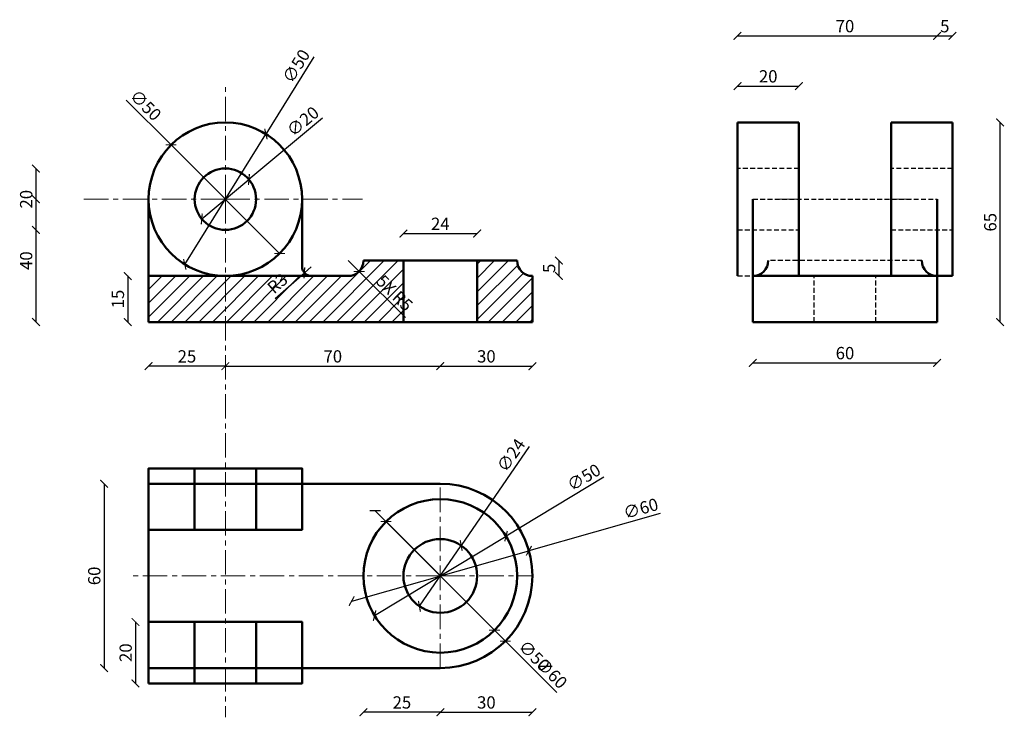
# Model space of a CAD drawing. Units: millimetres. Extents: x 2989 to 6790, y 1383 to 3069.
# Tile 1 of 1: x 2989.2 to 3309.8, y 1383.2 to 1610.3. Entities that reach past the tile are written whole.
import ezdxf

# ---------------------------------------------------------------- set-up
doc = ezdxf.new("R2010")
doc.units = ezdxf.units.MM
doc.header["$LTSCALE"] = 0.25
doc.linetypes.add('CENTER', pattern=[50.8, 31.75, -6.35, 6.35, -6.35])
doc.linetypes.add('HIDDEN', pattern=[9.525, 6.35, -3.175])
for name, color, linetype, lineweight in [('M-CNTR', 1, 'CENTER', 18), ('M-DIMS', 2, 'Continuous', 25), ('M-HATC', 8, 'Continuous', 18), ('M-HIDN', 6, 'HIDDEN', 25), ('M-OUTL', 7, 'Continuous', 50)]:
    doc.layers.add(name, color=color, linetype=linetype, lineweight=lineweight)
doc.styles.get("Standard").update_dxf_attribs({"font": 'arial.ttf'})
doc.dimstyles.new('ISO-25', dxfattribs={"dimtxt": 4, "dimasz": 2.5, "dimexe": 1.25, "dimexo": 0.625, "dimtad": 1, "dimdec": 0, "dimtxsty": 'Standard', "dimblk": 'ARCHTICK', "dimcen": 2.5, "dimse1": 1, "dimse2": 1, "dimadec": 0, "dimazin": 0, "dimtfac": 1, "dimtdec": 0, "dimtmove": 0, "dimatfit": 3, "dimfxl": 1, "dimarcsym": 0})

# ---------------------------------------------------------------- blocks, each defined once
blk = doc.blocks.new('_ArchTick')
at = {"color": 0, "linetype": 'ByBlock', "const_width": 0.15}
blk.add_lwpolyline([(-0.5, -0.5), (0.5, 0.5)], dxfattribs=at)
blk = doc.blocks.new('*D1')
at = {"layer": 'Defpoints', "color": 0, "transparency": 16777216}
for p in [(3126.13, 1429.2), (3156.13, 1429.2), (3156.13, 1384.81)]:
    blk.add_point(p, dxfattribs=at)
at = {"layer": 'M-DIMS', "color": 0, "lineweight": -2, "transparency": 16777216}
blk.add_line((3126.13, 1384.81), (3156.13, 1384.81), dxfattribs=at)
at = {"layer": 'M-DIMS', "color": 0, "lineweight": -2, "transparency": 16777216, "xscale": 2.5, "yscale": 2.5, "zscale": 2.5, "rotation": 180}
blk.add_blockref('_ArchTick', (3126.13, 1384.81), dxfattribs=at)
at = {"layer": 'M-DIMS', "color": 0, "lineweight": -2, "transparency": 16777216, "xscale": 2.5, "yscale": 2.5, "zscale": 2.5}
blk.add_blockref('_ArchTick', (3156.13, 1384.81), dxfattribs=at)
at = {"layer": 'M-DIMS', "color": 0, "transparency": 16777216, "insert": (3141.13, 1387.48), "char_height": 4, "attachment_point": 5}
blk.add_mtext('30', dxfattribs=at)
blk = doc.blocks.new('*D2')
at = {"layer": 'Defpoints', "color": 0, "transparency": 16777216}
for p in [(3126.13, 1511.85), (3156.13, 1511.85), (3156.13, 1497.49)]:
    blk.add_point(p, dxfattribs=at)
at = {"layer": 'M-DIMS', "color": 0, "lineweight": -2, "transparency": 16777216}
blk.add_line((3126.13, 1497.49), (3156.13, 1497.49), dxfattribs=at)
at = {"layer": 'M-DIMS', "color": 0, "lineweight": -2, "transparency": 16777216, "xscale": 2.5, "yscale": 2.5, "zscale": 2.5, "rotation": 180}
blk.add_blockref('_ArchTick', (3126.13, 1497.49), dxfattribs=at)
at = {"layer": 'M-DIMS', "color": 0, "lineweight": -2, "transparency": 16777216, "xscale": 2.5, "yscale": 2.5, "zscale": 2.5}
blk.add_blockref('_ArchTick', (3156.13, 1497.49), dxfattribs=at)
at = {"layer": 'M-DIMS', "color": 0, "transparency": 16777216, "insert": (3141.13, 1500.16), "char_height": 4, "attachment_point": 5}
blk.add_mtext('30', dxfattribs=at)
blk = doc.blocks.new('*D3')
at = {"layer": 'Defpoints', "color": 0, "transparency": 16777216}
for p in [(3031.13, 1511.85), (3056.13, 1511.85), (3031.13, 1497.49)]:
    blk.add_point(p, dxfattribs=at)
at = {"layer": 'M-DIMS', "color": 0, "lineweight": -2, "transparency": 16777216}
blk.add_line((3056.13, 1497.49), (3031.13, 1497.49), dxfattribs=at)
at = {"layer": 'M-DIMS', "color": 0, "lineweight": -2, "transparency": 16777216, "xscale": 2.5, "yscale": 2.5, "zscale": 2.5, "rotation": 180}
blk.add_blockref('_ArchTick', (3031.13, 1497.49), dxfattribs=at)
at = {"layer": 'M-DIMS', "color": 0, "lineweight": -2, "transparency": 16777216, "xscale": 2.5, "yscale": 2.5, "zscale": 2.5}
blk.add_blockref('_ArchTick', (3056.13, 1497.49), dxfattribs=at)
at = {"layer": 'M-DIMS', "color": 0, "transparency": 16777216, "insert": (3043.63, 1500.16), "char_height": 4, "attachment_point": 5}
blk.add_mtext('25', dxfattribs=at)
blk = doc.blocks.new('*D4')
at = {"layer": 'Defpoints', "color": 0, "transparency": 16777216}
for p in [(3056.13, 1511.85), (3126.13, 1511.85), (3126.13, 1497.49)]:
    blk.add_point(p, dxfattribs=at)
at = {"layer": 'M-DIMS', "color": 0, "lineweight": -2, "transparency": 16777216}
blk.add_line((3056.13, 1497.49), (3126.13, 1497.49), dxfattribs=at)
at = {"layer": 'M-DIMS', "color": 0, "lineweight": -2, "transparency": 16777216, "xscale": 2.5, "yscale": 2.5, "zscale": 2.5, "rotation": 180}
blk.add_blockref('_ArchTick', (3056.13, 1497.49), dxfattribs=at)
at = {"layer": 'M-DIMS', "color": 0, "lineweight": -2, "transparency": 16777216, "xscale": 2.5, "yscale": 2.5, "zscale": 2.5}
blk.add_blockref('_ArchTick', (3126.13, 1497.49), dxfattribs=at)
at = {"layer": 'M-DIMS', "color": 0, "transparency": 16777216, "insert": (3091.13, 1500.16), "char_height": 4, "attachment_point": 5}
blk.add_mtext('70', dxfattribs=at)
blk = doc.blocks.new('*D6')
at = {"layer": 'Defpoints', "color": 0, "transparency": 16777216}
for p in [(3101.13, 1429.2), (3126.13, 1429.2), (3101.13, 1384.81)]:
    blk.add_point(p, dxfattribs=at)
at = {"layer": 'M-DIMS', "color": 0, "lineweight": -2, "transparency": 16777216}
blk.add_line((3126.13, 1384.81), (3101.13, 1384.81), dxfattribs=at)
at = {"layer": 'M-DIMS', "color": 0, "lineweight": -2, "transparency": 16777216, "xscale": 2.5, "yscale": 2.5, "zscale": 2.5, "rotation": 180}
blk.add_blockref('_ArchTick', (3101.13, 1384.81), dxfattribs=at)
at = {"layer": 'M-DIMS', "color": 0, "lineweight": -2, "transparency": 16777216, "xscale": 2.5, "yscale": 2.5, "zscale": 2.5}
blk.add_blockref('_ArchTick', (3126.13, 1384.81), dxfattribs=at)
at = {"layer": 'M-DIMS', "color": 0, "transparency": 16777216, "insert": (3113.63, 1387.48), "char_height": 4, "attachment_point": 5}
blk.add_mtext('25', dxfattribs=at)
blk = doc.blocks.new('*D7')
at = {"layer": 'Defpoints', "color": 0, "transparency": 16777216}
for p in [(3138.13, 1540.69), (3114.13, 1531.85), (3138.13, 1531.85)]:
    blk.add_point(p, dxfattribs=at)
at = {"layer": 'M-DIMS', "color": 0, "lineweight": -2, "transparency": 16777216}
blk.add_line((3114.13, 1540.69), (3138.13, 1540.69), dxfattribs=at)
at = {"layer": 'M-DIMS', "color": 0, "lineweight": -2, "transparency": 16777216, "xscale": 2.5, "yscale": 2.5, "zscale": 2.5, "rotation": 180}
blk.add_blockref('_ArchTick', (3114.13, 1540.69), dxfattribs=at)
at = {"layer": 'M-DIMS', "color": 0, "lineweight": -2, "transparency": 16777216, "xscale": 2.5, "yscale": 2.5, "zscale": 2.5}
blk.add_blockref('_ArchTick', (3138.13, 1540.69), dxfattribs=at)
at = {"layer": 'M-DIMS', "color": 0, "transparency": 16777216, "insert": (3126.13, 1543.32), "char_height": 4, "attachment_point": 5}
blk.add_mtext('24', dxfattribs=at)
blk = doc.blocks.new('*D8')
at = {"layer": 'Defpoints', "color": 0, "transparency": 16777216}
for p in [(3063.81, 1558.26), (3048.45, 1545.44)]:
    blk.add_point(p, dxfattribs=at)
at = {"layer": 'M-DIMS', "color": 0, "lineweight": -2, "transparency": 16777216}
for p in [(3087.82, 1578.29), (3048.45, 1545.44)]:
    blk.add_line(p, (3063.81, 1558.26), dxfattribs=at)
at = {"layer": 'M-DIMS', "color": 0, "lineweight": -2, "transparency": 16777216, "xscale": 2.5, "yscale": 2.5, "zscale": 2.5}
for p, rotation in [((3063.81, 1558.26), 219.8399543782543), ((3048.45, 1545.44), 39.83995437825426)]:
    blk.add_blockref('_ArchTick', p, dxfattribs=dict(at, rotation=rotation))
at = {"layer": 'M-DIMS', "color": 0, "transparency": 16777216, "insert": (3081.69, 1576.8), "char_height": 4, "attachment_point": 5, "rotation": 39.84}
blk.add_mtext('∅20', dxfattribs=at)
blk = doc.blocks.new('*D9')
at = {"layer": 'Defpoints', "color": 0, "transparency": 16777216}
for p in [(3069.34, 1573.08), (3042.92, 1530.62)]:
    blk.add_point(p, dxfattribs=at)
at = {"layer": 'M-DIMS', "color": 0, "lineweight": -2, "transparency": 16777216}
for p in [(3084.99, 1598.24), (3042.92, 1530.62)]:
    blk.add_line(p, (3069.34, 1573.08), dxfattribs=at)
at = {"layer": 'M-DIMS', "color": 0, "lineweight": -2, "transparency": 16777216, "xscale": 2.5, "yscale": 2.5, "zscale": 2.5}
for p, rotation in [((3069.34, 1573.08), 238.1130736025114), ((3042.92, 1530.62), 58.11307360251142)]:
    blk.add_blockref('_ArchTick', p, dxfattribs=dict(at, rotation=rotation))
at = {"layer": 'M-DIMS', "color": 0, "transparency": 16777216, "insert": (3079.64, 1594.91), "char_height": 4, "attachment_point": 5, "rotation": 58.1131}
blk.add_mtext('∅50', dxfattribs=at)
blk = doc.blocks.new('*D10')
at = {"layer": 'Defpoints', "color": 0, "transparency": 16777216}
for p in [(3132.93, 1439.09), (3119.33, 1419.32)]:
    blk.add_point(p, dxfattribs=at)
at = {"layer": 'M-DIMS', "color": 0, "lineweight": -2, "transparency": 16777216}
for p in [(3155.09, 1471.29), (3119.33, 1419.32)]:
    blk.add_line(p, (3132.93, 1439.09), dxfattribs=at)
at = {"layer": 'M-DIMS', "color": 0, "lineweight": -2, "transparency": 16777216, "xscale": 2.5, "yscale": 2.5, "zscale": 2.5}
for p, rotation in [((3132.93, 1439.09), 235.4688788951653), ((3119.33, 1419.32), 55.46887889516527)]:
    blk.add_blockref('_ArchTick', p, dxfattribs=dict(at, rotation=rotation))
at = {"layer": 'M-DIMS', "color": 0, "transparency": 16777216, "insert": (3149.59, 1468.2), "char_height": 4, "attachment_point": 5, "rotation": 55.4689}
blk.add_mtext('∅24', dxfattribs=at)
blk = doc.blocks.new('*D11')
at = {"layer": 'Defpoints', "color": 0, "transparency": 16777216}
for p in [(3147.53, 1442.13), (3104.73, 1416.28)]:
    blk.add_point(p, dxfattribs=at)
at = {"layer": 'M-DIMS', "color": 0, "lineweight": -2, "transparency": 16777216}
for p in [(3179.41, 1461.38), (3104.73, 1416.28)]:
    blk.add_line(p, (3147.53, 1442.13), dxfattribs=at)
at = {"layer": 'M-DIMS', "color": 0, "lineweight": -2, "transparency": 16777216, "xscale": 2.5, "yscale": 2.5, "zscale": 2.5}
for p, rotation in [((3147.53, 1442.13), 211.1310054605087), ((3104.73, 1416.28), 31.13100546050863)]:
    blk.add_blockref('_ArchTick', p, dxfattribs=dict(at, rotation=rotation))
at = {"layer": 'M-DIMS', "color": 0, "transparency": 16777216, "insert": (3173.13, 1460.84), "char_height": 4, "attachment_point": 5, "rotation": 31.131}
blk.add_mtext('∅50', dxfattribs=at)
blk = doc.blocks.new('*D12')
at = {"layer": 'Defpoints', "color": 0, "transparency": 16777216}
for p in [(3154.99, 1437.39), (3097.27, 1421.02)]:
    blk.add_point(p, dxfattribs=at)
at = {"layer": 'M-DIMS', "color": 0, "lineweight": -2, "transparency": 16777216}
for p in [(3197.75, 1449.52), (3097.27, 1421.02)]:
    blk.add_line(p, (3154.99, 1437.39), dxfattribs=at)
at = {"layer": 'M-DIMS', "color": 0, "lineweight": -2, "transparency": 16777216, "xscale": 2.5, "yscale": 2.5, "zscale": 2.5}
for p, rotation in [((3154.99, 1437.39), 195.8331089062419), ((3097.27, 1421.02), 15.83310890624199)]:
    blk.add_blockref('_ArchTick', p, dxfattribs=dict(at, rotation=rotation))
at = {"layer": 'M-DIMS', "color": 0, "transparency": 16777216, "insert": (3191.55, 1450.65), "char_height": 4, "attachment_point": 5, "rotation": 15.8331}
blk.add_mtext('∅60', dxfattribs=at)
blk = doc.blocks.new('*D13')
at = {"layer": 'Defpoints', "color": 0, "transparency": 16777216}
for p in [(3031.13, 1459.2), (3016.63, 1399.2), (3031.13, 1399.2)]:
    blk.add_point(p, dxfattribs=at)
at = {"layer": 'M-DIMS', "color": 0, "lineweight": -2, "transparency": 16777216}
blk.add_line((3016.63, 1459.2), (3016.63, 1399.2), dxfattribs=at)
at = {"layer": 'M-DIMS', "color": 0, "lineweight": -2, "transparency": 16777216, "xscale": 2.5, "yscale": 2.5, "zscale": 2.5}
for p, rotation in [((3016.63, 1459.2), 90), ((3016.63, 1399.2), 270)]:
    blk.add_blockref('_ArchTick', p, dxfattribs=dict(at, rotation=rotation))
at = {"layer": 'M-DIMS', "color": 0, "transparency": 16777216, "insert": (3013.96, 1429.2), "char_height": 4, "attachment_point": 5, "rotation": 90}
blk.add_mtext('60', dxfattribs=at)
blk = doc.blocks.new('*D14')
at = {"layer": 'Defpoints', "color": 0, "transparency": 16777216}
for p in [(3031.13, 1414.2), (3026.86, 1394.2), (3031.13, 1394.2)]:
    blk.add_point(p, dxfattribs=at)
at = {"layer": 'M-DIMS', "color": 0, "lineweight": -2, "transparency": 16777216}
blk.add_line((3026.86, 1414.2), (3026.86, 1394.2), dxfattribs=at)
at = {"layer": 'M-DIMS', "color": 0, "lineweight": -2, "transparency": 16777216, "xscale": 2.5, "yscale": 2.5, "zscale": 2.5}
for p, rotation in [((3026.86, 1414.2), 90), ((3026.86, 1394.2), 270)]:
    blk.add_blockref('_ArchTick', p, dxfattribs=dict(at, rotation=rotation))
at = {"layer": 'M-DIMS', "color": 0, "transparency": 16777216, "insert": (3024.19, 1404.2), "char_height": 4, "attachment_point": 5, "rotation": 90}
blk.add_mtext('20', dxfattribs=at)
blk = doc.blocks.new('*D15')
at = {"layer": 'Defpoints', "color": 0, "transparency": 16777216}
for p in [(3031.13, 1526.85), (3024.33, 1511.85), (3031.13, 1511.85)]:
    blk.add_point(p, dxfattribs=at)
at = {"layer": 'M-DIMS', "color": 0, "lineweight": -2, "transparency": 16777216}
blk.add_line((3024.33, 1526.85), (3024.33, 1511.85), dxfattribs=at)
at = {"layer": 'M-DIMS', "color": 0, "lineweight": -2, "transparency": 16777216, "xscale": 2.5, "yscale": 2.5, "zscale": 2.5}
for p, rotation in [((3024.33, 1526.85), 90), ((3024.33, 1511.85), 270)]:
    blk.add_blockref('_ArchTick', p, dxfattribs=dict(at, rotation=rotation))
at = {"layer": 'M-DIMS', "color": 0, "transparency": 16777216, "insert": (3021.66, 1519.35), "char_height": 4, "attachment_point": 5, "rotation": 90}
blk.add_mtext('15', dxfattribs=at)
blk = doc.blocks.new('*D16')
at = {"layer": 'Defpoints', "color": 0, "transparency": 16777216}
for p in [(3227.91, 1511.85), (3287.91, 1511.85), (3287.91, 1498.56)]:
    blk.add_point(p, dxfattribs=at)
at = {"layer": 'M-DIMS', "color": 0, "lineweight": -2, "transparency": 16777216}
blk.add_line((3227.91, 1498.56), (3287.91, 1498.56), dxfattribs=at)
at = {"layer": 'M-DIMS', "color": 0, "lineweight": -2, "transparency": 16777216, "xscale": 2.5, "yscale": 2.5, "zscale": 2.5, "rotation": 180}
blk.add_blockref('_ArchTick', (3227.91, 1498.56), dxfattribs=at)
at = {"layer": 'M-DIMS', "color": 0, "lineweight": -2, "transparency": 16777216, "xscale": 2.5, "yscale": 2.5, "zscale": 2.5}
blk.add_blockref('_ArchTick', (3287.91, 1498.56), dxfattribs=at)
at = {"layer": 'M-DIMS', "color": 0, "transparency": 16777216, "insert": (3257.91, 1501.22), "char_height": 4, "attachment_point": 5}
blk.add_mtext('60', dxfattribs=at)
blk = doc.blocks.new('*D17')
at = {"layer": 'Defpoints', "color": 0, "transparency": 16777216}
for p in [(3242.91, 1588.68), (3222.91, 1576.85), (3242.91, 1576.85)]:
    blk.add_point(p, dxfattribs=at)
at = {"layer": 'M-DIMS', "color": 0, "lineweight": -2, "transparency": 16777216}
blk.add_line((3222.91, 1588.68), (3242.91, 1588.68), dxfattribs=at)
at = {"layer": 'M-DIMS', "color": 0, "lineweight": -2, "transparency": 16777216, "xscale": 2.5, "yscale": 2.5, "zscale": 2.5, "rotation": 180}
blk.add_blockref('_ArchTick', (3222.91, 1588.68), dxfattribs=at)
at = {"layer": 'M-DIMS', "color": 0, "lineweight": -2, "transparency": 16777216, "xscale": 2.5, "yscale": 2.5, "zscale": 2.5}
blk.add_blockref('_ArchTick', (3242.91, 1588.68), dxfattribs=at)
at = {"layer": 'M-DIMS', "color": 0, "transparency": 16777216, "insert": (3232.91, 1591.34), "char_height": 4, "attachment_point": 5}
blk.add_mtext('20', dxfattribs=at)
blk = doc.blocks.new('*D18')
at = {"layer": 'Defpoints', "color": 0, "transparency": 16777216}
for p in [(3151.13, 1531.85), (3156.13, 1526.85), (3164.74, 1526.85)]:
    blk.add_point(p, dxfattribs=at)
at = {"layer": 'M-DIMS', "color": 0, "lineweight": -2, "transparency": 16777216}
blk.add_line((3164.74, 1531.85), (3164.74, 1526.85), dxfattribs=at)
at = {"layer": 'M-DIMS', "color": 0, "lineweight": -2, "transparency": 16777216, "xscale": 2.5, "yscale": 2.5, "zscale": 2.5}
for p, rotation in [((3164.74, 1531.85), 90), ((3164.74, 1526.85), 270)]:
    blk.add_blockref('_ArchTick', p, dxfattribs=dict(at, rotation=rotation))
at = {"layer": 'M-DIMS', "color": 0, "transparency": 16777216, "insert": (3162.08, 1529.35), "char_height": 4, "attachment_point": 5, "rotation": 90}
blk.add_mtext('5', dxfattribs=at)
blk = doc.blocks.new('*D19')
at = {"layer": 'Defpoints', "color": 0, "transparency": 16777216}
for p in [(3031.13, 1551.85), (2994.45, 1511.85), (3031.13, 1511.85)]:
    blk.add_point(p, dxfattribs=at)
at = {"layer": 'M-DIMS', "color": 0, "lineweight": -2, "transparency": 16777216}
blk.add_line((2994.45, 1551.85), (2994.45, 1511.85), dxfattribs=at)
at = {"layer": 'M-DIMS', "color": 0, "lineweight": -2, "transparency": 16777216, "xscale": 2.5, "yscale": 2.5, "zscale": 2.5}
for p, rotation in [((2994.45, 1551.85), 90), ((2994.45, 1511.85), 270)]:
    blk.add_blockref('_ArchTick', p, dxfattribs=dict(at, rotation=rotation))
at = {"layer": 'M-DIMS', "color": 0, "transparency": 16777216, "insert": (2991.79, 1531.85), "char_height": 4, "attachment_point": 5, "rotation": 90}
blk.add_mtext('40', dxfattribs=at)
blk = doc.blocks.new('*D20')
at = {"layer": 'Defpoints', "color": 0, "transparency": 16777216}
for p in [(3292.91, 1576.85), (3308.41, 1576.85), (3287.91, 1511.85)]:
    blk.add_point(p, dxfattribs=at)
at = {"layer": 'M-DIMS', "color": 0, "lineweight": -2, "transparency": 16777216}
blk.add_line((3308.41, 1511.85), (3308.41, 1576.85), dxfattribs=at)
at = {"layer": 'M-DIMS', "color": 0, "lineweight": -2, "transparency": 16777216, "xscale": 2.5, "yscale": 2.5, "zscale": 2.5}
for p, rotation in [((3308.41, 1576.85), 90), ((3308.41, 1511.85), 270)]:
    blk.add_blockref('_ArchTick', p, dxfattribs=dict(at, rotation=rotation))
at = {"layer": 'M-DIMS', "color": 0, "transparency": 16777216, "insert": (3305.74, 1544.35), "char_height": 4, "attachment_point": 5, "rotation": 90}
blk.add_mtext('65', dxfattribs=at)
blk = doc.blocks.new('*D21')
at = {"layer": 'Defpoints', "color": 0, "transparency": 16777216}
for p in [(3292.91, 1605.01), (3222.91, 1576.85), (3292.91, 1576.85)]:
    blk.add_point(p, dxfattribs=at)
at = {"layer": 'M-DIMS', "color": 0, "lineweight": -2, "transparency": 16777216}
blk.add_line((3222.91, 1605.01), (3292.91, 1605.01), dxfattribs=at)
at = {"layer": 'M-DIMS', "color": 0, "lineweight": -2, "transparency": 16777216, "xscale": 2.5, "yscale": 2.5, "zscale": 2.5, "rotation": 180}
blk.add_blockref('_ArchTick', (3222.91, 1605.01), dxfattribs=at)
at = {"layer": 'M-DIMS', "color": 0, "lineweight": -2, "transparency": 16777216, "xscale": 2.5, "yscale": 2.5, "zscale": 2.5}
blk.add_blockref('_ArchTick', (3292.91, 1605.01), dxfattribs=at)
at = {"layer": 'M-DIMS', "color": 0, "transparency": 16777216, "insert": (3257.91, 1607.68), "char_height": 4, "attachment_point": 5}
blk.add_mtext('70', dxfattribs=at)
blk = doc.blocks.new('*D22')
at = {"layer": 'Defpoints', "color": 0, "transparency": 16777216}
for p in [(3222.91, 1561.85), (2994.45, 1541.85), (3222.91, 1541.85)]:
    blk.add_point(p, dxfattribs=at)
at = {"layer": 'M-DIMS', "color": 0, "lineweight": -2, "transparency": 16777216}
blk.add_line((2994.45, 1561.85), (2994.45, 1541.85), dxfattribs=at)
at = {"layer": 'M-DIMS', "color": 0, "lineweight": -2, "transparency": 16777216, "xscale": 2.5, "yscale": 2.5, "zscale": 2.5}
for p, rotation in [((2994.45, 1561.85), 90), ((2994.45, 1541.85), 270)]:
    blk.add_blockref('_ArchTick', p, dxfattribs=dict(at, rotation=rotation))
at = {"layer": 'M-DIMS', "color": 0, "transparency": 16777216, "insert": (2991.79, 1551.85), "char_height": 4, "attachment_point": 5, "rotation": 90}
blk.add_mtext('20', dxfattribs=at)
blk = doc.blocks.new('*D23')
at = {"layer": 'Defpoints', "color": 0, "transparency": 16777216}
for p in [(3292.91, 1605.01), (3287.91, 1526.85), (3292.91, 1526.85)]:
    blk.add_point(p, dxfattribs=at)
at = {"layer": 'M-DIMS', "color": 0, "lineweight": -2, "transparency": 16777216}
blk.add_line((3287.91, 1605.01), (3292.91, 1605.01), dxfattribs=at)
at = {"layer": 'M-DIMS', "color": 0, "lineweight": -2, "transparency": 16777216, "xscale": 2.5, "yscale": 2.5, "zscale": 2.5, "rotation": 180}
blk.add_blockref('_ArchTick', (3287.91, 1605.01), dxfattribs=at)
at = {"layer": 'M-DIMS', "color": 0, "lineweight": -2, "transparency": 16777216, "xscale": 2.5, "yscale": 2.5, "zscale": 2.5}
blk.add_blockref('_ArchTick', (3292.91, 1605.01), dxfattribs=at)
at = {"layer": 'M-DIMS', "color": 0, "transparency": 16777216, "insert": (3290.41, 1607.67), "char_height": 4, "attachment_point": 5}
blk.add_mtext('5', dxfattribs=at)
blk = doc.blocks.new('*D24')
at = {"layer": 'Defpoints', "color": 0, "transparency": 16777216}
for p in [(3038.45, 1569.53), (3073.81, 1534.17)]:
    blk.add_point(p, dxfattribs=at)
at = {"layer": 'M-DIMS', "color": 0, "lineweight": -2, "transparency": 16777216}
for p in [(3023.85, 1584.14), (3073.81, 1534.17)]:
    blk.add_line(p, (3038.45, 1569.53), dxfattribs=at)
at = {"layer": 'M-DIMS', "color": 0, "lineweight": -2, "transparency": 16777216, "xscale": 2.5, "yscale": 2.5, "zscale": 2.5}
for p, rotation in [((3038.45, 1569.53), 314.997023014067), ((3073.81, 1534.17), 134.997023014067)]:
    blk.add_blockref('_ArchTick', p, dxfattribs=dict(at, rotation=rotation))
at = {"layer": 'M-DIMS', "color": 0, "transparency": 16777216, "insert": (3029.81, 1582.1), "char_height": 4, "attachment_point": 5, "rotation": 314.997}
blk.add_mtext('∅50', dxfattribs=at)
blk = doc.blocks.new('*D25')
at = {"layer": 'Defpoints', "color": 0, "transparency": 16777216}
for p in [(3108.47, 1446.9), (3143.79, 1411.51)]:
    blk.add_point(p, dxfattribs=at)
at = {"layer": 'M-DIMS', "color": 0, "lineweight": -2, "transparency": 16777216}
for p in [(3108.47, 1446.9), (3158.39, 1396.89)]:
    blk.add_line(p, (3143.79, 1411.51), dxfattribs=at)
at = {"layer": 'M-DIMS', "color": 0, "lineweight": -2, "transparency": 16777216, "xscale": 2.5, "yscale": 2.5, "zscale": 2.5}
for p, rotation in [((3108.47, 1446.9), 314.9472925942576), ((3143.79, 1411.51), 134.9472925942575)]:
    blk.add_blockref('_ArchTick', p, dxfattribs=dict(at, rotation=rotation))
at = {"layer": 'M-DIMS', "color": 0, "transparency": 16777216, "insert": (3156.35, 1402.86), "char_height": 4, "attachment_point": 5, "rotation": 314.9473}
blk.add_mtext('∅50', dxfattribs=at)
blk = doc.blocks.new('*D26')
at = {"layer": 'Defpoints', "color": 0, "transparency": 16777216}
for p in [(3104.93, 1450.43), (3147.33, 1407.97)]:
    blk.add_point(p, dxfattribs=at)
at = {"layer": 'M-DIMS', "color": 0, "lineweight": -2, "transparency": 16777216}
for p in [(3104.93, 1450.43), (3164.04, 1391.23)]:
    blk.add_line(p, (3147.33, 1407.97), dxfattribs=at)
at = {"layer": 'M-DIMS', "color": 0, "lineweight": -2, "transparency": 16777216, "xscale": 2.5, "yscale": 2.5, "zscale": 2.5}
for p, rotation in [((3104.93, 1450.43), 314.9560015369301), ((3147.33, 1407.97), 134.9560015369301)]:
    blk.add_blockref('_ArchTick', p, dxfattribs=dict(at, rotation=rotation))
at = {"layer": 'M-DIMS', "color": 0, "transparency": 16777216, "insert": (3162.01, 1397.2), "char_height": 4, "attachment_point": 5, "rotation": 314.956}
blk.add_mtext('∅60', dxfattribs=at)
blk = doc.blocks.new('*D27')
at = {"layer": 'Defpoints', "color": 0, "transparency": 16777216}
for p in [(3096.13, 1531.85), (3099.68, 1528.32)]:
    blk.add_point(p, dxfattribs=at)
at = {"layer": 'M-DIMS', "color": 0, "lineweight": -2, "transparency": 16777216}
for p in [(3096.13, 1531.85), (3114.8, 1513.29)]:
    blk.add_line(p, (3099.68, 1528.32), dxfattribs=at)
at = {"layer": 'M-DIMS', "color": 0, "lineweight": -2, "transparency": 16777216, "xscale": 2.5, "yscale": 2.5, "zscale": 2.5, "rotation": 135.1757510372473}
blk.add_blockref('_ArchTick', (3099.68, 1528.32), dxfattribs=at)
at = {"layer": 'M-DIMS', "color": 0, "transparency": 16777216, "insert": (3110.89, 1520.93), "char_height": 4, "attachment_point": 5, "rotation": 315.1758}
blk.add_mtext('5X R5', dxfattribs=at)
blk = doc.blocks.new('*D28')
at = {"layer": 'Defpoints', "color": 0, "transparency": 16777216}
for p in [(3084.13, 1529.85), (3081.87, 1527.87)]:
    blk.add_point(p, dxfattribs=at)
at = {"layer": 'M-DIMS', "color": 0, "lineweight": -2, "transparency": 16777216}
for p in [(3084.13, 1529.85), (3072.31, 1519.52)]:
    blk.add_line(p, (3081.87, 1527.87), dxfattribs=at)
at = {"layer": 'M-DIMS', "color": 0, "lineweight": -2, "transparency": 16777216, "xscale": 2.5, "yscale": 2.5, "zscale": 2.5, "rotation": 41.15405449249937}
blk.add_blockref('_ArchTick', (3081.87, 1527.87), dxfattribs=at)
at = {"layer": 'M-DIMS', "color": 0, "transparency": 16777216, "insert": (3073.45, 1524.06), "char_height": 4, "attachment_point": 5, "rotation": 41.1541}
blk.add_mtext('R3', dxfattribs=at)

msp = doc.modelspace()

# ---------------------------------------------------------------- hatches: boundary and pattern name
at = {"layer": 'M-HATC'}
h = msp.add_hatch(dxfattribs=at)
h.set_pattern_fill('ANSI31', color=256)
h.paths.add_polyline_path([(3114.13, 1531.85), (3101.13, 1531.85, -0.414214), (3096.13, 1526.85), (3084.13, 1526.85), (3056.13, 1526.85), (3056.13, 1511.85), (3114.13, 1511.85)])
h.paths.add_polyline_path([(3056.13, 1526.85), (3031.13, 1526.85), (3031.13, 1511.85), (3056.13, 1511.85)])
h.paths.add_polyline_path([(3156.13, 1526.85, -0.414214), (3151.13, 1531.85), (3138.13, 1531.85), (3138.13, 1511.85), (3156.13, 1511.85)])

# ---------------------------------------------------------------- linework, layer by layer
at = {"layer": 'M-CNTR'}
for p, q in [((3056.13, 1551.85), (3056.13, 1589.51)), ((3056.13, 1551.85), (3009.95, 1551.85)), ((3056.13, 1551.85), (3056.13, 1383.16)), ((3056.13, 1551.85), (3100.84, 1551.85)), ((3242.91, 1551.85), (3236.16, 1551.85)), ((3279.62, 1551.85), (3272.91, 1551.85)), ((3126.13, 1399.2), (3126.13, 1459.2)), ((3126.13, 1429.2), (3024.79, 1429.2)), ((3126.13, 1429.2), (3156.13, 1429.2))]:
    msp.add_line(p, q, dxfattribs=at)
at = {"layer": 'M-HIDN'}
for p, q in [((3242.91, 1561.85), (3222.91, 1561.85)), ((3292.91, 1561.85), (3272.91, 1561.85)), ((3227.91, 1551.85), (3287.91, 1551.85)), ((3222.91, 1541.85), (3242.91, 1541.85)), ((3272.91, 1541.85), (3292.91, 1541.85)), ((3282.91, 1531.85), (3232.91, 1531.85)), ((3222.91, 1526.85), (3242.91, 1526.85)), ((3247.91, 1511.85), (3247.91, 1526.85)), ((3267.91, 1511.85), (3267.91, 1526.85)), ((3272.91, 1526.85), (3287.91, 1526.85))]:
    msp.add_line(p, q, dxfattribs=at)
at = {"layer": 'M-OUTL'}
for p, q in [((3242.91, 1576.85), (3222.91, 1576.85)), ((3222.91, 1576.85), (3222.91, 1526.85)), ((3242.91, 1526.85), (3242.91, 1576.85)), ((3292.91, 1576.85), (3272.91, 1576.85)), ((3272.91, 1576.85), (3272.91, 1526.85)), ((3292.91, 1526.85), (3292.91, 1576.85)), ((3031.13, 1526.85), (3031.13, 1551.85)), ((3081.13, 1551.85), (3081.13, 1529.85)), ((3227.91, 1526.85), (3227.91, 1551.85)), ((3287.91, 1551.85), (3287.91, 1541.85)), ((3287.91, 1541.85), (3287.91, 1526.85)), ((3126.13, 1531.85), (3101.13, 1531.85)), ((3101.13, 1531.85), (3101.13, 1531.85)), ((3114.13, 1531.85), (3114.13, 1511.85)), ((3126.13, 1531.85), (3151.13, 1531.85)), ((3138.13, 1531.85), (3138.13, 1511.85)), ((3227.91, 1531.85), (3227.91, 1531.85)), ((3031.13, 1511.85), (3031.13, 1526.85)), ((3086.13, 1526.85), (3031.13, 1526.85)), ((3084.13, 1526.85), (3096.13, 1526.85)), ((3156.13, 1511.85), (3156.13, 1526.85)), ((3222.91, 1526.85), (3222.91, 1526.85)), ((3287.91, 1526.85), (3227.91, 1526.85)), ((3227.91, 1526.85), (3227.91, 1511.85)), ((3227.91, 1526.85), (3227.91, 1526.85)), ((3287.91, 1511.85), (3287.91, 1526.85)), ((3287.91, 1526.85), (3292.91, 1526.85)), ((3292.91, 1526.85), (3292.91, 1526.85)), ((3031.13, 1511.85), (3056.13, 1511.85)), ((3056.13, 1511.85), (3126.13, 1511.85)), ((3138.13, 1511.85), (3126.13, 1511.85)), ((3138.13, 1511.85), (3156.13, 1511.85)), ((3227.91, 1511.85), (3287.91, 1511.85)), ((3046.13, 1464.2), (3046.13, 1444.2)), ((3066.13, 1464.2), (3066.13, 1444.2)), ((3031.13, 1459.2), (3031.13, 1399.2)), ((3126.13, 1459.2), (3031.13, 1459.2)), ((3046.13, 1414.2), (3046.13, 1394.2)), ((3066.13, 1414.2), (3066.13, 1394.2)), ((3031.13, 1399.2), (3056.13, 1399.2)), ((3056.13, 1399.2), (3126.13, 1399.2))]:
    msp.add_line(p, q, dxfattribs=at)
for points in [[(3031.13, 1444.2), (3081.13, 1444.2), (3081.13, 1464.2), (3031.13, 1464.2)], [(3031.13, 1394.2), (3081.13, 1394.2), (3081.13, 1414.2), (3031.13, 1414.2)]]:
    msp.add_lwpolyline(points, close=True, dxfattribs=at)
for centre, radius in [((3056.13, 1551.85), 25), ((3056.13, 1551.85), 10), ((3126.13, 1429.2), 25), ((3126.13, 1429.2), 12)]:
    msp.add_circle(centre, radius, dxfattribs=at)
for centre, radius, start, end in [((3084.13, 1529.85), 3, 180, 270), ((3096.13, 1531.85), 5, 270, 0), ((3156.13, 1531.85), 5, 180, 270), ((3227.91, 1531.85), 5, 270, 0), ((3287.91, 1531.85), 5, 180, 270), ((3126.13, 1429.2), 30, 270, 90)]:
    msp.add_arc(centre, radius, start, end, dxfattribs=at)

# ---------------------------------------------------------------- dimensions: what is measured, and where the dimension line sits
at = {"layer": 'M-DIMS'}
for base, p1, p2, override, picture, middle in [((3292.91, 1605.01), (3222.91, 1576.85), (3292.91, 1576.85), {"dimdec": 0, "dimlfac": 1, "dimrnd": 0, "dimzin": 0, "dimdsep": 46, "dimlunit": 2}, '*D21', (3257.91, 1607.68)), ((3292.91, 1605.01), (3287.91, 1526.85), (3292.91, 1526.85), {"dimdec": 0, "dimlfac": 1, "dimrnd": 0, "dimzin": 0, "dimdsep": 46, "dimlunit": 2}, '*D23', (3290.41, 1607.67)), ((3242.91, 1588.68), (3222.91, 1576.85), (3242.91, 1576.85), {"dimclrd": 0, "dimclre": 0, "dimclrt": 0}, '*D17', (3232.91, 1591.34)), ((3138.13, 1540.69), (3114.13, 1531.85), (3138.13, 1531.85), {"dimclrd": 0, "dimclre": 0, "dimclrt": 0}, '*D7', (3126.13, 1543.32)), ((3031.13, 1497.49), (3056.13, 1511.85), (3031.13, 1511.85), {"dimclrd": 0, "dimclre": 0, "dimclrt": 0}, '*D3', (3043.63, 1500.16)), ((3126.13, 1497.49), (3056.13, 1511.85), (3126.13, 1511.85), {"dimclrd": 0, "dimclre": 0, "dimclrt": 0}, '*D4', (3091.13, 1500.16)), ((3156.13, 1497.49), (3126.13, 1511.85), (3156.13, 1511.85), {"dimclrd": 0, "dimclre": 0, "dimclrt": 0}, '*D2', (3141.13, 1500.16)), ((3287.91, 1498.56), (3227.91, 1511.85), (3287.91, 1511.85), {"dimclrd": 0, "dimclre": 0, "dimclrt": 0}, '*D16', (3257.91, 1501.22)), ((3101.13, 1384.81), (3126.13, 1429.2), (3101.13, 1429.2), {"dimclrd": 0, "dimclre": 0, "dimclrt": 0}, '*D6', (3113.63, 1387.48)), ((3156.13, 1384.81), (3126.13, 1429.2), (3156.13, 1429.2), {"dimclrd": 0, "dimclre": 0, "dimclrt": 0}, '*D1', (3141.13, 1387.48))]:
    dim = msp.add_linear_dim(base=base, p1=p1, p2=p2, dimstyle='ISO-25', override=override, dxfattribs=at)
    dim.commit()
    dim.dimension.update_dxf_attribs({"geometry": picture, "text_midpoint": middle})
for p1, p2, override, picture, middle in [((3042.92, 1530.62), (3069.34, 1573.08), {"dimclrd": 0, "dimclre": 0, "dimclrt": 0}, '*D9', (3082, 1593.44)), ((3073.81, 1534.17), (3038.45, 1569.53), {"dimdec": 0, "dimlfac": 1, "dimrnd": 0, "dimzin": 0, "dimdsep": 46, "dimlunit": 2}, '*D24', (3027.85, 1580.13)), ((3048.45, 1545.44), (3063.81, 1558.26), {"dimclrd": 0, "dimclre": 0, "dimclrt": 0}, '*D8', (3083.47, 1574.66)), ((3119.33, 1419.32), (3132.93, 1439.09), {"dimclrd": 0, "dimclre": 0, "dimclrt": 0}, '*D10', (3151.88, 1466.63)), ((3104.73, 1416.28), (3147.53, 1442.13), {"dimclrd": 0, "dimclre": 0, "dimclrt": 0}, '*D11', (3174.56, 1458.46)), ((3097.27, 1421.02), (3154.99, 1437.39), {"dimclrd": 0, "dimclre": 0, "dimclrt": 0}, '*D12', (3192.31, 1447.97)), ((3104.93, 1450.43), (3147.33, 1407.97), {"dimdec": 0, "dimlfac": 1, "dimrnd": 0, "dimzin": 0, "dimdsep": 46, "dimlunit": 2}, '*D26', (3160.04, 1395.24)), ((3108.47, 1446.9), (3143.79, 1411.51), {"dimdec": 0, "dimlfac": 1, "dimrnd": 0, "dimzin": 0, "dimdsep": 46, "dimlunit": 2}, '*D25', (3154.39, 1400.89))]:
    dim = msp.add_diameter_dim_2p(p1=p1, p2=p2, dimstyle='ISO-25', override=override, dxfattribs=at)
    dim.commit()
    dim.dimension.update_dxf_attribs({"geometry": picture, "text_midpoint": middle, "dimtype": 163})
for base, p1, p2, override, picture, middle in [((3308.41, 1576.85), (3287.91, 1511.85), (3292.91, 1576.85), {"dimdec": 0, "dimlfac": 1, "dimrnd": 0, "dimzin": 0, "dimdsep": 46, "dimlunit": 2}, '*D20', (3305.74, 1544.35)), ((2994.45, 1541.85), (3222.91, 1561.85), (3222.91, 1541.85), {"dimdec": 0, "dimlfac": 1, "dimrnd": 0, "dimzin": 0, "dimdsep": 46, "dimlunit": 2}, '*D22', (2991.79, 1551.85)), ((2994.45, 1511.85), (3031.13, 1551.85), (3031.13, 1511.85), {"dimdec": 0, "dimlfac": 1, "dimrnd": 0, "dimzin": 0, "dimdsep": 46, "dimlunit": 2}, '*D19', (2991.79, 1531.85)), ((3164.74, 1526.85), (3151.13, 1531.85), (3156.13, 1526.85), {"dimclrd": 0, "dimclre": 0, "dimclrt": 0}, '*D18', (3162.08, 1529.35)), ((3024.33, 1511.85), (3031.13, 1526.85), (3031.13, 1511.85), {"dimclrd": 0, "dimclre": 0, "dimclrt": 0}, '*D15', (3021.66, 1519.35)), ((3016.63, 1399.2), (3031.13, 1459.2), (3031.13, 1399.2), {"dimclrd": 0, "dimclre": 0, "dimclrt": 0}, '*D13', (3013.96, 1429.2)), ((3026.86, 1394.2), (3031.13, 1414.2), (3031.13, 1394.2), {"dimclrd": 0, "dimclre": 0, "dimclrt": 0}, '*D14', (3024.19, 1404.2))]:
    dim = msp.add_linear_dim(base=base, p1=p1, p2=p2, angle=90, dimstyle='ISO-25', override=override, dxfattribs=at)
    dim.commit()
    dim.dimension.update_dxf_attribs({"geometry": picture, "text_midpoint": middle})
dim = msp.add_radius_dim(center=(3084.13, 1529.85), mpoint=(3081.87, 1527.87), dimstyle='ISO-25', override={"dimdec": 0, "dimlfac": 1, "dimrnd": 0, "dimzin": 0, "dimdsep": 46, "dimlunit": 2}, dxfattribs=at)
dim.commit()
dim.dimension.update_dxf_attribs({"geometry": '*D28', "text_midpoint": (3073.45, 1524.06)})
dim = msp.add_radius_dim(center=(3096.13, 1531.85), mpoint=(3099.68, 1528.32), text='5X <>', dimstyle='ISO-25', override={"dimdec": 0, "dimlfac": 1, "dimrnd": 0, "dimzin": 0, "dimdsep": 46, "dimlunit": 2}, dxfattribs=at)
dim.commit()
dim.dimension.update_dxf_attribs({"geometry": '*D27', "text_midpoint": (3110.89, 1520.93)})

doc.saveas('drawing.dxf')
